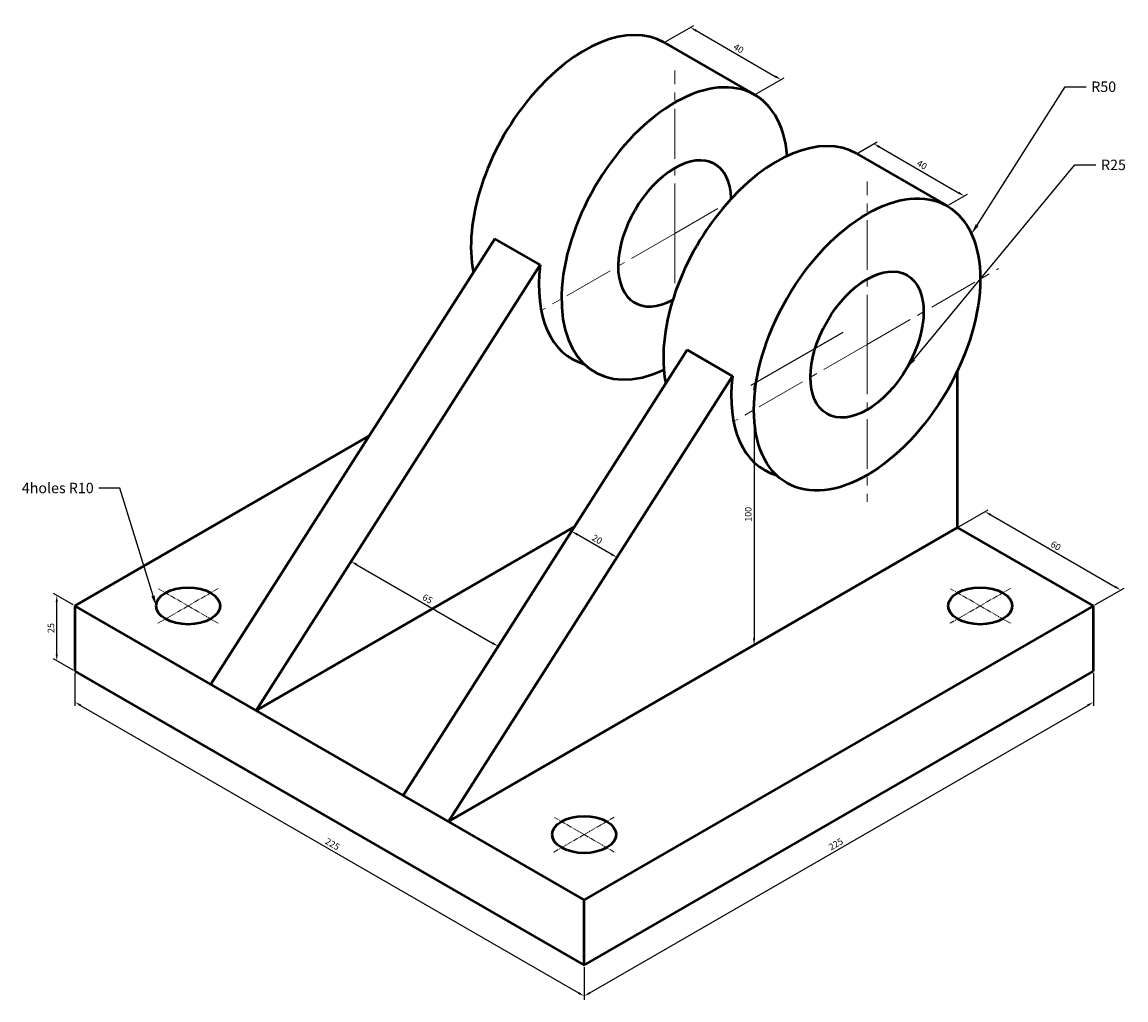
# Model space of a CAD drawing. Units: millimetres. Extents: x 2471 to 2893, y 1618 to 1992.
import ezdxf
from ezdxf import colors
from ezdxf.entities.mleader import LeaderData, LeaderLine
from ezdxf.math import Vec2, Vec3

# ---------------------------------------------------------------- set-up
doc = ezdxf.new("R2010")
doc.units = ezdxf.units.MM
doc.linetypes.add('CENTER2', pattern=[28.575, 19.05, -3.175, 3.175, -3.175])
for name, color, linetype, lineweight in [('M-CNTR', 1, 'CENTER2', 18), ('M-DIMS', 2, 'Continuous', 25), ('M-OUTL', 7, 'Continuous', 50)]:
    doc.layers.add(name, color=color, linetype=linetype, lineweight=lineweight)
doc.styles.get("Standard").update_dxf_attribs({"font": 'arial.ttf'})
doc.dimstyles.new('ISO-25', dxfattribs={"dimtxt": 2.5, "dimasz": 2.5, "dimexe": 1.25, "dimexo": 0.625, "dimtad": 1, "dimtxsty": 'Standard', "dimcen": 2.5, "dimadec": 0, "dimazin": 0, "dimtfac": 1, "dimtmove": 0, "dimatfit": 3, "dimfxl": 1, "dimarcsym": 0})

# ---------------------------------------------------------------- blocks, each defined once
blk = doc.blocks.new('*D1')
at = {"layer": 'Defpoints', "color": 0, "transparency": 16777216}
for p in [(2491.04, 1743.51), (2685.89, 1631.01), (2685.89, 1619.2)]:
    blk.add_point(p, dxfattribs=at)
at = {"layer": 'M-DIMS', "color": 0, "lineweight": -2, "transparency": 16777216}
for p, q in [((2491.04, 1742.79), (2491.04, 1730.25)), ((2493.2, 1730.45), (2683.73, 1620.45)), ((2685.89, 1630.29), (2685.89, 1617.75))]:
    blk.add_line(p, q, dxfattribs=at)
at = {"layer": 'M-DIMS', "color": 0, "transparency": 16777216}
for points in [[(2493.41, 1730.81), (2492.99, 1730.09), (2491.04, 1731.7)], [(2683.94, 1620.81), (2683.52, 1620.09), (2685.89, 1619.2)]]:
    blk.add_solid(points, dxfattribs=at)
at = {"layer": 'M-DIMS', "color": 0, "transparency": 16777216, "insert": (2589.42, 1677.09), "char_height": 2.5, "attachment_point": 5, "rotation": 330}
blk.add_mtext('225', dxfattribs=at)
blk = doc.blocks.new('*D2')
at = {"layer": 'Defpoints', "color": 0, "transparency": 16777216}
for p in [(2484.07, 1772.54), (2491.04, 1768.51), (2491.04, 1743.51)]:
    blk.add_point(p, dxfattribs=at)
at = {"layer": 'M-DIMS', "color": 0, "lineweight": -2, "transparency": 16777216}
for p, q in [((2490.41, 1768.87), (2482.82, 1773.26)), ((2484.07, 1750.04), (2484.07, 1770.04)), ((2490.41, 1743.87), (2482.82, 1748.26))]:
    blk.add_line(p, q, dxfattribs=at)
at = {"layer": 'M-DIMS', "color": 0, "transparency": 16777216}
for points in [[(2483.65, 1770.04), (2484.48, 1770.04), (2484.07, 1772.54)], [(2483.65, 1750.04), (2484.48, 1750.04), (2484.07, 1747.54)]]:
    blk.add_solid(points, dxfattribs=at)
at = {"layer": 'M-DIMS', "color": 0, "transparency": 16777216, "insert": (2482.17, 1760.04), "char_height": 2.5, "attachment_point": 5, "rotation": 90}
blk.add_mtext('25', dxfattribs=at)
blk = doc.blocks.new('*D3')
at = {"layer": 'Defpoints', "color": 0, "transparency": 16777216}
for p in [(2880.75, 1743.51), (2880.75, 1731.7), (2685.89, 1631.01)]:
    blk.add_point(p, dxfattribs=at)
at = {"layer": 'M-DIMS', "color": 0, "lineweight": -2, "transparency": 16777216}
for p, q in [((2880.75, 1742.79), (2880.75, 1730.25)), ((2688.06, 1620.45), (2878.58, 1730.45)), ((2685.89, 1630.29), (2685.89, 1617.75))]:
    blk.add_line(p, q, dxfattribs=at)
at = {"layer": 'M-DIMS', "color": 0, "transparency": 16777216}
for points in [[(2878.37, 1730.81), (2878.79, 1730.09), (2880.75, 1731.7)], [(2687.85, 1620.81), (2688.27, 1620.09), (2685.89, 1619.2)]]:
    blk.add_solid(points, dxfattribs=at)
at = {"layer": 'M-DIMS', "color": 0, "transparency": 16777216, "insert": (2782.37, 1677.09), "char_height": 2.5, "attachment_point": 5, "rotation": 30}
blk.add_mtext('225', dxfattribs=at)
blk = doc.blocks.new('*D4')
at = {"layer": 'Defpoints', "color": 0, "transparency": 16777216}
for p in [(2828.79, 1798.51), (2891.25, 1774.58), (2880.75, 1768.51)]:
    blk.add_point(p, dxfattribs=at)
at = {"layer": 'M-DIMS', "color": 0, "lineweight": -2, "transparency": 16777216}
for p, q in [((2829.41, 1798.87), (2840.54, 1805.3)), ((2841.46, 1803.33), (2889.09, 1775.83)), ((2881.37, 1768.87), (2892.5, 1775.3))]:
    blk.add_line(p, q, dxfattribs=at)
at = {"layer": 'M-DIMS', "color": 0, "transparency": 16777216}
for points in [[(2841.67, 1803.69), (2841.25, 1802.97), (2839.29, 1804.58)], [(2889.3, 1776.19), (2888.88, 1775.47), (2891.25, 1774.58)]]:
    blk.add_solid(points, dxfattribs=at)
at = {"layer": 'M-DIMS', "color": 0, "transparency": 16777216, "insert": (2866.22, 1791.23), "char_height": 2.5, "attachment_point": 5, "rotation": 330}
blk.add_mtext('60', dxfattribs=at)
blk = doc.blocks.new('*D5')
at = {"layer": 'Defpoints', "color": 0, "transparency": 16777216}
for p in [(2680.73, 1796.49), (2681.09, 1797.06), (2698.05, 1786.49)]:
    blk.add_point(p, dxfattribs=at)
at = {"layer": 'M-DIMS', "color": 0, "lineweight": -2, "transparency": 16777216}
for p, q in [((2681.07, 1797.02), (2681.76, 1798.11)), ((2696.24, 1788.31), (2683.25, 1795.81)), ((2698.39, 1787.02), (2699.08, 1788.11))]:
    blk.add_line(p, q, dxfattribs=at)
at = {"layer": 'M-DIMS', "color": 0, "transparency": 16777216}
for points in [[(2683.46, 1796.17), (2683.04, 1795.45), (2681.09, 1797.06)], [(2696.45, 1788.67), (2696.04, 1787.95), (2698.41, 1787.06)]]:
    blk.add_solid(points, dxfattribs=at)
at = {"layer": 'M-DIMS', "color": 0, "transparency": 16777216, "insert": (2690.7, 1793.7), "char_height": 2.5, "attachment_point": 5, "rotation": 330}
blk.add_mtext('20', dxfattribs=at)
blk = doc.blocks.new('*D6')
at = {"layer": 'Defpoints', "color": 0, "transparency": 16777216}
for p in [(2790.12, 1941.55), (2831.36, 1925.35), (2824.76, 1921.55)]:
    blk.add_point(p, dxfattribs=at)
at = {"layer": 'M-DIMS', "color": 0, "lineweight": -2, "transparency": 16777216}
for p, q in [((2790.75, 1941.91), (2797.97, 1946.08)), ((2798.88, 1944.1), (2829.19, 1926.6)), ((2825.39, 1921.91), (2832.61, 1926.08))]:
    blk.add_line(p, q, dxfattribs=at)
at = {"layer": 'M-DIMS', "color": 0, "transparency": 16777216}
for points in [[(2799.09, 1944.46), (2798.67, 1943.74), (2796.72, 1945.35)], [(2829.4, 1926.96), (2828.98, 1926.24), (2831.36, 1925.35)]]:
    blk.add_solid(points, dxfattribs=at)
at = {"layer": 'M-DIMS', "color": 0, "transparency": 16777216, "insert": (2814.99, 1937), "char_height": 2.5, "attachment_point": 5, "rotation": 330}
blk.add_mtext('40', dxfattribs=at)
blk = doc.blocks.new('*D7')
at = {"layer": 'Defpoints', "color": 0, "transparency": 16777216}
for p in [(2716.51, 1984.05), (2761.21, 1969.85), (2751.15, 1964.05)]:
    blk.add_point(p, dxfattribs=at)
at = {"layer": 'M-DIMS', "color": 0, "lineweight": -2, "transparency": 16777216}
for p, q in [((2717.14, 1984.41), (2727.82, 1990.57)), ((2728.73, 1988.6), (2759.04, 1971.1)), ((2751.78, 1964.41), (2762.46, 1970.57))]:
    blk.add_line(p, q, dxfattribs=at)
at = {"layer": 'M-DIMS', "color": 0, "transparency": 16777216}
for points in [[(2728.94, 1988.96), (2728.52, 1988.24), (2726.57, 1989.85)], [(2759.25, 1971.46), (2758.83, 1970.74), (2761.21, 1969.85)]]:
    blk.add_solid(points, dxfattribs=at)
at = {"layer": 'M-DIMS', "color": 0, "transparency": 16777216, "insert": (2744.84, 1981.5), "char_height": 2.5, "attachment_point": 5, "rotation": 330}
blk.add_mtext('40', dxfattribs=at)
blk = doc.blocks.new('*D8')
at = {"layer": 'Defpoints', "color": 0, "transparency": 16777216}
for p in [(2653, 1753.03), (2560.32, 1728.51), (2616.61, 1696.01)]:
    blk.add_point(p, dxfattribs=at)
at = {"layer": 'M-DIMS', "color": 0, "lineweight": -2, "transparency": 16777216}
for p, q in [((2560.66, 1729.04), (2597.38, 1786.59)), ((2598.87, 1784.28), (2650.83, 1754.28)), ((2616.95, 1696.54), (2653.67, 1754.09))]:
    blk.add_line(p, q, dxfattribs=at)
at = {"layer": 'M-DIMS', "color": 0, "transparency": 16777216}
for points in [[(2599.08, 1784.64), (2598.66, 1783.92), (2596.7, 1785.53)], [(2651.04, 1754.64), (2650.62, 1753.92), (2653, 1753.03)]]:
    blk.add_solid(points, dxfattribs=at)
at = {"layer": 'M-DIMS', "color": 0, "transparency": 16777216, "insert": (2625.8, 1770.93), "char_height": 2.5, "attachment_point": 5, "rotation": 330}
blk.add_mtext('65', dxfattribs=at)
blk = doc.blocks.new('*D9')
at = {"layer": 'Defpoints', "color": 0, "transparency": 16777216}
for p in [(2785.49, 1873.51), (2785.49, 1773.51), (2750.91, 1753.55)]:
    blk.add_point(p, dxfattribs=at)
at = {"layer": 'M-DIMS', "color": 0, "lineweight": -2, "transparency": 16777216}
for p, q in [((2784.86, 1873.15), (2749.66, 1852.83)), ((2750.91, 1851.05), (2750.91, 1756.05)), ((2784.86, 1773.15), (2749.66, 1752.83))]:
    blk.add_line(p, q, dxfattribs=at)
at = {"layer": 'M-DIMS', "color": 0, "transparency": 16777216}
for points in [[(2750.5, 1851.05), (2751.33, 1851.05), (2750.91, 1853.55)], [(2750.5, 1756.05), (2751.33, 1756.05), (2750.91, 1753.55)]]:
    blk.add_solid(points, dxfattribs=at)
at = {"layer": 'M-DIMS', "color": 0, "transparency": 16777216, "insert": (2749.01, 1803.55), "char_height": 2.5, "attachment_point": 5, "rotation": 90}
blk.add_mtext('100', dxfattribs=at)
blk = doc.blocks.new('CENTER-MARK-HOLE')
at = {"ltscale": 0.1}
for q in [(0.46, 13.4), (23.66, 13.66), (0, 0), (23.66, 0)]:
    blk.add_line((11.83, 6.83), q, dxfattribs=at)

msp = doc.modelspace()

# ---------------------------------------------------------------- linework, layer by layer
at = {"layer": 'M-CNTR'}
for p, q in [((2720.533, 1911.014), (2720.533, 1973.381)), ((2794.145, 1868.514), (2794.145, 1930.881)), ((2720.533, 1911.014), (2740.63, 1922.616)), ((2720.533, 1911.014), (2670.177, 1881.941)), ((2720.533, 1911.014), (2720.533, 1887.808)), ((2794.145, 1868.514), (2844.415, 1897.537)), ((2794.145, 1868.514), (2743.79, 1839.441)), ((2794.145, 1868.514), (2794.145, 1808.299))]:
    msp.add_line(p, q, dxfattribs=at)
at = {"layer": 'M-OUTL'}
for p, q in [((2716.511, 1984.047), (2751.152, 1964.047)), ((2790.123, 1941.547), (2824.764, 1921.547)), ((2651.761, 1908.955), (2542.998, 1738.514)), ((2669.081, 1898.955), (2651.761, 1908.955)), ((2669.081, 1898.955), (2560.319, 1728.514)), ((2725.373, 1866.455), (2616.61, 1696.014)), ((2742.693, 1856.455), (2725.373, 1866.455)), ((2742.693, 1856.455), (2633.931, 1686.014)), ((2828.786, 1798.514), (2828.786, 1858.514)), ((2491.037, 1768.514), (2603.62, 1833.514)), ((2560.319, 1728.514), (2682.284, 1798.93)), ((2828.786, 1798.514), (2633.931, 1686.014)), ((2880.748, 1768.514), (2828.786, 1798.514)), ((2685.892, 1656.014), (2491.037, 1768.514)), ((2491.037, 1768.514), (2491.037, 1743.514)), ((2880.748, 1768.514), (2685.892, 1656.014)), ((2880.748, 1743.514), (2880.748, 1768.514)), ((2491.037, 1743.514), (2685.892, 1631.014)), ((2685.892, 1631.014), (2880.748, 1743.514)), ((2685.892, 1631.014), (2685.892, 1656.014))]:
    msp.add_line(p, q, dxfattribs=at)
for centre, major_axis, start_param, end_param in [((2685.892, 1931.014), (-30.619, -53.033), 3.1415927, 5.7088942), ((2720.533, 1911.014), (-30.619, -53.033), 2.4517756, 6.9730024), ((2759.504, 1888.514), (-30.619, -53.033), 3.1415927, 5.7088942), ((2720.533, 1911.014), (-15.309, -26.517), 2.3889958, 7.0357822), ((2711.873, 1916.014), (-30.619, -53.033), 5.3442434, 6.4250824), ((2785.485, 1873.514), (-30.619, -53.033), 5.3442434, 6.4250824)]:
    msp.add_ellipse(centre, major_axis=major_axis, ratio=0.5773503, start_param=start_param, end_param=end_param, dxfattribs=at)
for centre, major_axis in [((2794.145, 1868.514), (-30.619, -53.033)), ((2794.145, 1868.514), (-15.309, -26.517)), ((2534.338, 1768.514), (-12.247, 0)), ((2837.447, 1768.514), (-12.247, 0)), ((2685.892, 1681.014), (-12.247, 0))]:
    msp.add_ellipse(centre, major_axis=major_axis, ratio=0.5773503, dxfattribs=at)

# ---------------------------------------------------------------- block references
at = {"layer": 'M-CNTR'}
for p in [(2522.506, 1761.683), (2825.615, 1761.683), (2674.061, 1674.183)]:
    msp.add_blockref('CENTER-MARK-HOLE', p, dxfattribs=at)

# ---------------------------------------------------------------- dimensions: what is measured, and where the dimension line sits
at = {"layer": 'M-DIMS'}
for p1, p2, distance, picture, middle in [((2716.511, 1984.047), (2751.152, 1964.047), 10.054, '*D7', (2744.836, 1981.498)), ((2790.123, 1941.547), (2824.764, 1921.547), 6.593, '*D6', (2814.988, 1937)), ((2785.485, 1873.514), (2785.485, 1773.514), -34.573, '*D9', (2749.01, 1803.553)), ((2828.786, 1798.514), (2880.748, 1768.514), 10.506, '*D4', (2866.224, 1791.226)), ((2698.05, 1786.495), (2680.729, 1796.495), -0.666, '*D5', (2690.699, 1793.703)), ((2560.319, 1728.514), (2616.61, 1696.014), 67.573, '*D8', (2625.801, 1770.93)), ((2491.037, 1743.514), (2491.037, 1768.514), 6.969, '*D2', (2482.166, 1760.037)), ((2491.037, 1743.514), (2685.892, 1631.014), -10.235, '*D1', (2589.415, 1677.093)), ((2685.892, 1631.014), (2880.748, 1743.514), -10.235, '*D3', (2782.369, 1677.093))]:
    dim = msp.add_aligned_dim(p1=p1, p2=p2, distance=distance, dimstyle='ISO-25', override={"dimclrd": 0, "dimclre": 0, "dimclrt": 0}, dxfattribs=at)
    dim.commit()
    dim.dimension.update_dxf_attribs({"geometry": picture, "text_midpoint": middle})

# ---------------------------------------------------------------- leaders
ml = msp.add_multileader_mtext('Standard', dxfattribs=at)
ml.set_content('R50', color=256)
ml.set_leader_properties()
ml.build(insert=Vec2(0, 0))
ctx = ml.context
ctx.base_point, ctx.plane_origin = Vec3(2877.951, 1967.114), Vec3(2834.113, 1910.828)
notes = []
notes.append((ctx, [(0, (1, 1, 0), (2869.951, 1967.114), (1, 0), 8, [(0, [(2834.113, 1910.828)], 0, [])])]))
ctx.mtext.insert, ctx.mtext.flow_direction = Vec3(2879.951, 1969.148), 5
ml = msp.add_multileader_mtext('Standard', dxfattribs=at)
ml.set_content('R25', color=256)
ml.set_leader_properties()
ml.build(insert=Vec2(0, 0))
ctx = ml.context
ctx.base_point, ctx.plane_origin = Vec3(2881.693, 1937.206), Vec3(2809.455, 1859.675)
notes.append((ctx, [(0, (1, 1, 0), (2873.693, 1937.206), (1, 0), 8, [(0, [(2809.455, 1859.675)], 0, [])])]))
ctx.mtext.insert, ctx.mtext.flow_direction = Vec3(2883.693, 1939.24), 5
ml = msp.add_multileader_mtext('Standard', dxfattribs=at)
ml.set_content('4holes R10', color=256)
ml.set_leader_properties()
ml.build(insert=Vec2(0, 0))
ctx = ml.context
ctx.base_point, ctx.plane_origin = Vec3(2468.276, 1813.586), Vec3(2522.09, 1768.514)
ctx.text_align_type = 2
notes.append((ctx, [(0, (1, 1, 0), (2508.208, 1813.586), (-1, 0), 8, [(0, [(2522.09, 1768.514)], 0, [])])]))
ctx.mtext.insert, ctx.mtext.alignment, ctx.mtext.flow_direction = Vec3(2498.208, 1815.621), 3, 5
for ctx, leaders in notes:
    for number, flags, end, landing, length, lines in leaders:
        leader = LeaderData()
        leader.index, (leader.has_last_leader_line, leader.has_dogleg_vector, leader.attachment_direction) = number, flags
        leader.last_leader_point, leader.dogleg_vector, leader.dogleg_length = Vec3(end), Vec3(landing), length
        for number, points, colour, breaks in lines:
            line = LeaderLine()
            line.index, line.vertices, line.color, line.breaks = number, Vec3.list(points), colors.encode_raw_color(colour), breaks
            leader.lines.append(line)
        ctx.leaders.append(leader)

doc.saveas('drawing.dxf')
